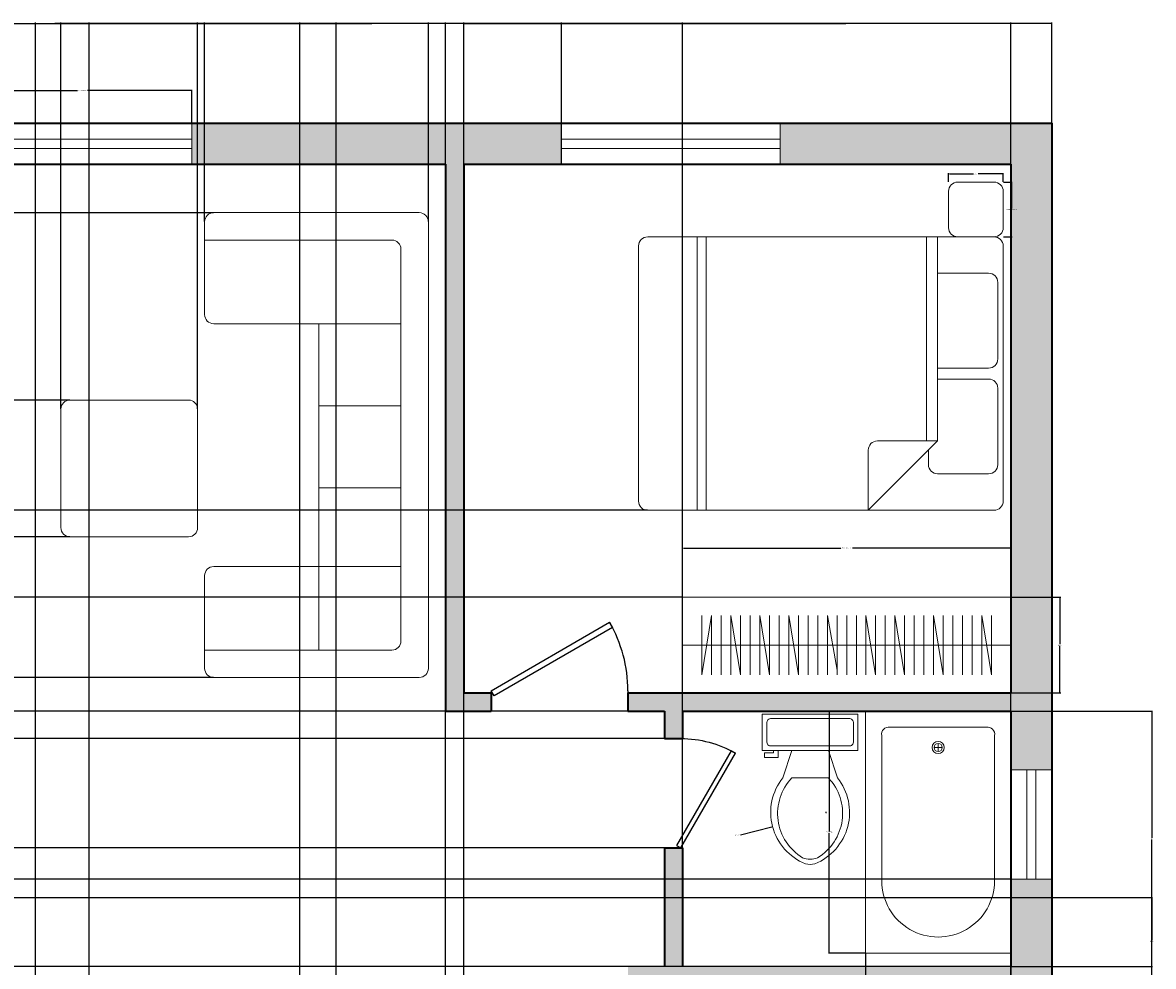
# Model space of a CAD drawing. Units: inches. Extents: x 2800 to 3283, y 1752 to 2114.
# Tile 6 of 6: x 3035 to 3283, y 1907 to 2114. Entities that reach past the tile are written whole.
import ezdxf

# ---------------------------------------------------------------- set-up
doc = ezdxf.new("R2010")
doc.units = ezdxf.units.IN
for name, color, linetype, lineweight in [('A-ANNO-DIMS', 2, 'Continuous', 18), ('A-DOOR', 3, 'Continuous', 25), ('A-FLOR-CASE', 8, 'Continuous', 18), ('A-FLOR-FIXT', 9, 'Continuous', 18), ('A-FURN', 9, 'Continuous', 18), ('A-GLAZ', 4, 'Continuous', 18), ('A-WALL', 7, 'Continuous', 35)]:
    doc.layers.add(name, color=color, linetype=linetype, lineweight=lineweight)
doc.layers.add('A-WALL-PATT', color=18, linetype='Continuous', lineweight=13, true_color=0x000000)
doc.styles.get("Standard").update_dxf_attribs({"font": 'arial.ttf'})
doc.dimstyles.get("Standard").update_dxf_attribs({"dimtxt": 0.18, "dimasz": 0.18, "dimexe": 0.18, "dimexo": 0.0625, "dimgap": 0.09, "dimtad": 0, "dimtih": 1, "dimtoh": 1, "dimdec": 4, "dimzin": 0, "dimdsep": 46, "dimtxsty": 'Standard', "dimcen": 0.09, "dimadec": 0, "dimazin": 0, "dimtfac": 1, "dimtdec": 4, "dimtofl": 0, "dimtmove": 0, "dimatfit": 3, "dimfxl": 1, "dimtolj": 1, "dimtzin": 0, "dimarcsym": 0})

# ---------------------------------------------------------------- blocks, each defined once
blk = doc.blocks.new('Bed - Queen')
for p, q in [((2, 0), (58, 0)), ((0, -78), (0, -2)), ((10, -1.2), (26.8, -1.2)), ((33.2, -1.2), (50, -1.2)), ((60, -2), (60, -78)), ((8, -14.4), (8, -3.2)), ((28.8, -3.2), (28.8, -14.4)), ((31.2, -14.4), (31.2, -3.2)), ((52, -3.2), (52, -14.4)), ((0, -14.4), (44.8, -14.4)), ((60, -29.6), (44.8, -14.4)), ((44.8, -14.4), (44.8, -27.6)), ((44.8, -16.8), (0, -16.8)), ((50, -16.4), (46.8, -16.4)), ((46.8, -29.6), (60, -29.6)), ((0, -65.18), (60, -65.18)), ((0, -67.18), (60, -67.18)), ((58, -80), (2, -80))]:
    blk.add_line(p, q)
for centre, start, end in [((58, -2), 0, 90), ((2, -2), 90, 180), ((10, -3.2), 90, 180), ((26.8, -3.2), 0, 90), ((33.2, -3.2), 90, 180), ((50, -3.2), 0, 90), ((50, -14.4), 270, 0), ((46.8, -27.6), 180, 270), ((2, -78), 180, 270), ((58, -78), 270, 0)]:
    blk.add_arc(centre, 2, start, end)
blk = doc.blocks.new('Bath Tub - 26 x 60 in.')
for p, q in [((8, -18), (10, -18)), ((9, -17), (9, -19))]:
    blk.add_line(p, q)
blk.add_lwpolyline([(0, -36), (0, 0), (60, 0), (60, -36)], close=True)
for points in [[(6, -4), (42, -4)], [(4, -30), (4, -6)], [(42, -32), (6, -32)]]:
    blk.add_lwpolyline(points)
for radius in [1.5, 1]:
    blk.add_circle((9, -18), radius)
for centre, radius, start, end in [((5.75, -5.75), 1.77, 81.8699, 188.1301), ((42, -18), 14, 270, 90), ((5.75, -30.25), 1.77, 171.8699, 278.1301)]:
    blk.add_arc(centre, radius, start, end)
blk = doc.blocks.new('Toilet - top')
for p, q in [((9.5, -6), (9.5, -2)), ((-10, -8.5), (-8, -8.5)), ((-10, -9.5), (-10, -8.5)), ((-7, -9.5), (-10, -9.5)), ((-8, -8.5), (-8, -8)), ((-7, -8), (-7, -9.5)), ((-4, -8), (-6, -14)), ((4, -8), (6, -14)), ((4, -14), (-4, -14))]:
    blk.add_line(p, q)
blk.add_lwpolyline([(10.5, -8), (10.5, 0), (-10.5, 0), (-10.5, -8)], close=True)
for points in [[(-9.5, -2), (-9.5, -6)], [(8.5, -1), (-8.5, -1)], [(-8.5, -7), (8.5, -7)]]:
    blk.add_lwpolyline(points)
for centre, radius, start, end in [((-8.62, -1.88), 0.884, 81.8699, 188.1301), ((8.62, -1.88), 0.884, 351.8699, 98.1301), ((-8.62, -6.12), 0.884, 171.8699, 278.1301), ((8.62, -6.12), 0.884, 261.8699, 8.1301), ((3.52, -21.58), 12.17, 141.4691, 247.9714), ((4.2, -21.82), 11.33, 136.3677, 238.9468), ((-3.52, -21.58), 12.17, 292.0284, 38.5307), ((-4.2, -21.82), 11.33, 301.053, 43.6321), ((0, -27.88), 4, 245.7318, 294.2682), ((0, -29), 4, 254.8605, 285.1395)]:
    blk.add_arc(centre, radius, start, end)
blk = doc.blocks.new('*U12')
for p, q in [((0, 0), (0, -6)), ((40, 0), (40, -6))]:
    blk.add_line(p, q)
blk.add_lwpolyline([(0, 0), (34.64, 20), (35.52, 18.48), (0.87, -1.52)], close=True)
blk.add_arc((0, 0), 40, 0, 30)
blk = doc.blocks.new('WARDROBE-72')
for p, q in [((10.5, 72), (10.5, 0)), ((17, 63.53), (4, 63.53)), ((17, 61.41), (4, 61.41)), ((17, 59.29), (4, 59.29)), ((17, 52.94), (4, 52.94)), ((17, 50.82), (4, 50.82)), ((17, 44.47), (4, 44.47)), ((17, 38.12), (4, 38.12)), ((17, 36), (4, 36)), ((17, 33.88), (4, 33.88)), ((17, 29.65), (4, 29.65)), ((17, 27.53), (4, 27.53)), ((17, 21.18), (4, 21.18)), ((17, 14.82), (4, 14.82)), ((17, 8.47), (4, 8.47))]:
    blk.add_line(p, q)
for points in [[(0, 0), (0, 72), (21, 72), (21, 0), (0, 0), (21, 0)], [(4, 67.76), (17, 67.76), (4, 65.65), (17, 65.65)], [(4, 57.18), (17, 57.18), (4, 55.06), (17, 55.06)], [(4, 48.71), (17, 48.71), (4, 46.59), (17, 46.59)], [(4, 42.35), (17, 42.35), (4, 40.23), (17, 40.23)], [(16.02, 33.88), (4, 31.76), (17, 31.76)], [(4, 25.41), (17, 25.41), (4, 23.29), (17, 23.29)], [(4, 19.06), (17, 19.06), (4, 16.94), (17, 16.94)], [(4, 12.71), (17, 12.71), (4, 10.59), (17, 10.59)], [(4, 4.23), (17, 4.23), (4, 6.35), (17, 6.35)]]:
    blk.add_lwpolyline(points)
blk = doc.blocks.new('WIN-48')
for p, q in [((0, 5.5), (48, 5.5)), ((0, 3.5), (48, 3.5))]:
    blk.add_line(p, q)
for points in [[(0, 0), (0, 9)], [(48, 9), (48, 0)]]:
    blk.add_lwpolyline(points)
blk = doc.blocks.new('WIN-24')
for p, q in [((3.5, 24), (3.5, 0)), ((5.5, 24), (5.5, 0))]:
    blk.add_line(p, q)
for points in [[(0, 24), (9, 24)], [(9, 0), (0, 0)]]:
    blk.add_lwpolyline(points)
blk = doc.blocks.new('NIGHTSTAND-12')
blk.add_lwpolyline([(2, 0), (10, 0, 0.414214), (12, 2), (12, 10, 0.414214), (10, 12), (2, 12, 0.414214), (0, 10), (0, 2, 0.414214)], format="xyb", close=True)
blk = doc.blocks.new('*D19')
at = {"layer": 'A-ANNO-DIMS', "color": 0, "lineweight": -2, "transparency": 16777216}
for p, q in [((3023.88, 2092.33), (3023.88, 2099.65)), ((3024.06, 2099.47), (3046.76, 2099.47)), ((3071.7, 2099.47), (3049, 2099.47)), ((3071.88, 2092.33), (3071.88, 2099.65))]:
    blk.add_line(p, q, dxfattribs=at)
at = {"layer": 'A-ANNO-DIMS', "color": 0, "transparency": 16777216}
for points in [[(3024.06, 2099.5), (3024.06, 2099.44), (3023.88, 2099.47)], [(3071.7, 2099.5), (3071.7, 2099.44), (3071.88, 2099.47)]]:
    blk.add_solid(points, dxfattribs=at)
at = {"layer": 'Defpoints', "color": 0, "transparency": 16777216}
for p in [(3023.88, 2099.47), (3023.88, 2092.27), (3071.88, 2092.27)]:
    blk.add_point(p, dxfattribs=at)
at = {"layer": 'A-ANNO-DIMS', "color": 0, "transparency": 16777216, "insert": (3047.88, 2099.47), "char_height": 0.18, "attachment_point": 5}
blk.add_mtext('\\A1;WINDOW 48 TYP.', dxfattribs=at)
blk = doc.blocks.new('*D25')
at = {"layer": 'A-ANNO-DIMS', "color": 0, "lineweight": -2, "transparency": 16777216}
for p, q in [((3179.54, 1988.33), (3179.54, 1999.25)), ((3179.72, 1999.07), (3214.24, 1999.07)), ((3251.36, 1999.07), (3216.85, 1999.07)), ((3251.54, 1988.33), (3251.54, 1999.25))]:
    blk.add_line(p, q, dxfattribs=at)
at = {"layer": 'A-ANNO-DIMS', "color": 0, "transparency": 16777216}
for points in [[(3179.72, 1999.1), (3179.72, 1999.04), (3179.54, 1999.07)], [(3251.36, 1999.1), (3251.36, 1999.04), (3251.54, 1999.07)]]:
    blk.add_solid(points, dxfattribs=at)
at = {"layer": 'Defpoints', "color": 0, "transparency": 16777216}
for p in [(3251.54, 1999.07), (3179.54, 1988.27), (3251.54, 1988.27)]:
    blk.add_point(p, dxfattribs=at)
at = {"layer": 'A-ANNO-DIMS', "color": 0, "transparency": 16777216, "insert": (3215.54, 1999.07), "char_height": 0.18, "attachment_point": 5}
blk.add_mtext('\\A1;WARDROBE 72 TYP.', dxfattribs=at)
blk = doc.blocks.new('*D26')
at = {"layer": 'A-ANNO-DIMS', "color": 0, "lineweight": -2, "transparency": 16777216}
for p, q in [((3251.61, 1988.27), (3262.52, 1988.27)), ((3262.34, 1988.09), (3262.34, 1977.95)), ((3262.34, 1967.45), (3262.34, 1977.59)), ((3251.61, 1967.27), (3262.52, 1967.27))]:
    blk.add_line(p, q, dxfattribs=at)
at = {"layer": 'A-ANNO-DIMS', "color": 0, "transparency": 16777216}
for points in [[(3262.31, 1988.09), (3262.37, 1988.09), (3262.34, 1988.27)], [(3262.31, 1967.45), (3262.37, 1967.45), (3262.34, 1967.27)]]:
    blk.add_solid(points, dxfattribs=at)
at = {"layer": 'Defpoints', "color": 0, "transparency": 16777216}
for p in [(3251.54, 1988.27), (3251.54, 1967.27), (3262.34, 1967.27)]:
    blk.add_point(p, dxfattribs=at)
at = {"layer": 'A-ANNO-DIMS', "color": 0, "transparency": 16777216, "insert": (3262.34, 1977.77), "char_height": 0.18, "attachment_point": 5}
blk.add_mtext('\\A1;21 TYP.', dxfattribs=at)
blk = doc.blocks.new('*D29')
at = {"layer": 'A-ANNO-DIMS', "color": 0, "lineweight": -2, "transparency": 16777216}
for p, q in [((3249.95, 2079.36), (3251.87, 2079.36)), ((3251.69, 2079.18), (3251.69, 2073.54)), ((3251.69, 2067.54), (3251.69, 2073.18)), ((3249.95, 2067.36), (3251.87, 2067.36))]:
    blk.add_line(p, q, dxfattribs=at)
at = {"layer": 'A-ANNO-DIMS', "color": 0, "transparency": 16777216}
for points in [[(3251.66, 2079.18), (3251.72, 2079.18), (3251.69, 2079.36)], [(3251.66, 2067.54), (3251.72, 2067.54), (3251.69, 2067.36)]]:
    blk.add_solid(points, dxfattribs=at)
at = {"layer": 'Defpoints', "color": 0, "transparency": 16777216}
for p in [(3249.89, 2079.36), (3251.69, 2079.36), (3249.89, 2067.36)]:
    blk.add_point(p, dxfattribs=at)
at = {"layer": 'A-ANNO-DIMS', "color": 0, "transparency": 16777216, "insert": (3251.69, 2073.36), "char_height": 0.18, "attachment_point": 5}
blk.add_mtext('\\A1;NIGHTSTAND 12 TYP.', dxfattribs=at)
blk = doc.blocks.new('*D30')
at = {"layer": 'A-ANNO-DIMS', "color": 0, "lineweight": -2, "transparency": 16777216}
for p, q in [((3237.89, 2079.42), (3237.89, 2081.34)), ((3238.07, 2081.16), (3243.37, 2081.16)), ((3249.71, 2081.16), (3244.41, 2081.16)), ((3249.89, 2079.42), (3249.89, 2081.34))]:
    blk.add_line(p, q, dxfattribs=at)
at = {"layer": 'A-ANNO-DIMS', "color": 0, "transparency": 16777216}
for points in [[(3238.07, 2081.19), (3238.07, 2081.13), (3237.89, 2081.16)], [(3249.71, 2081.19), (3249.71, 2081.13), (3249.89, 2081.16)]]:
    blk.add_solid(points, dxfattribs=at)
at = {"layer": 'Defpoints', "color": 0, "transparency": 16777216}
for p in [(3237.89, 2081.16), (3237.89, 2079.36), (3249.89, 2079.36)]:
    blk.add_point(p, dxfattribs=at)
at = {"layer": 'A-ANNO-DIMS', "color": 0, "transparency": 16777216, "insert": (3243.89, 2081.16), "char_height": 0.18, "attachment_point": 5}
blk.add_mtext('\\A1;12 TYP.', dxfattribs=at)
blk = doc.blocks.new('*D31')
at = {"layer": 'A-ANNO-DIMS', "color": 0, "lineweight": -2, "transparency": 16777216}
for p, q in [((3219.62, 1963.27), (3211.53, 1963.27)), ((3211.71, 1963.09), (3211.71, 1936.9)), ((3211.71, 1910.34), (3211.71, 1936.53)), ((3219.62, 1910.16), (3211.53, 1910.16))]:
    blk.add_line(p, q, dxfattribs=at)
at = {"layer": 'A-ANNO-DIMS', "color": 0, "transparency": 16777216}
for points in [[(3211.68, 1963.09), (3211.74, 1963.09), (3211.71, 1963.27)], [(3211.68, 1910.34), (3211.74, 1910.34), (3211.71, 1910.16)]]:
    blk.add_solid(points, dxfattribs=at)
at = {"layer": 'Defpoints', "color": 0, "transparency": 16777216}
for p in [(3219.68, 1963.27), (3211.71, 1910.16), (3219.68, 1910.16)]:
    blk.add_point(p, dxfattribs=at)
at = {"layer": 'A-ANNO-DIMS', "color": 0, "transparency": 16777216, "insert": (3211.71, 1936.72), "char_height": 0.18, "attachment_point": 5}
blk.add_mtext('\\A1;TUB 53 TYP.', dxfattribs=at)
blk = doc.blocks.new('*D32')
at = {"layer": 'A-ANNO-DIMS', "color": 0, "lineweight": -2, "transparency": 16777216}
for p, q in [((3219.68, 1910.1), (3219.68, 1902.02)), ((3251.54, 1910.1), (3251.54, 1902.02)), ((3219.86, 1902.2), (3235.08, 1902.2)), ((3251.36, 1902.2), (3236.14, 1902.2))]:
    blk.add_line(p, q, dxfattribs=at)
at = {"layer": 'A-ANNO-DIMS', "color": 0, "transparency": 16777216}
for points in [[(3219.86, 1902.23), (3219.86, 1902.17), (3219.68, 1902.2)], [(3251.36, 1902.23), (3251.36, 1902.17), (3251.54, 1902.2)]]:
    blk.add_solid(points, dxfattribs=at)
at = {"layer": 'Defpoints', "color": 0, "transparency": 16777216}
for p in [(3219.68, 1910.16), (3251.54, 1910.16), (3251.54, 1902.2)]:
    blk.add_point(p, dxfattribs=at)
at = {"layer": 'A-ANNO-DIMS', "color": 0, "transparency": 16777216, "insert": (3235.61, 1902.2), "char_height": 0.18, "attachment_point": 5}
blk.add_mtext('\\A1;32 TYP.', dxfattribs=at)
blk = doc.blocks.new('*D43')
at = {"layer": 'A-ANNO-DIMS', "color": 0, "lineweight": -2, "transparency": 16777216}
for p, q in [((2822.54, 2092.33), (2822.54, 2114.36)), ((2822.72, 2114.18), (3041.25, 2114.18)), ((3260.36, 2114.18), (3041.84, 2114.18)), ((3260.54, 2092.33), (3260.54, 2114.36))]:
    blk.add_line(p, q, dxfattribs=at)
at = {"layer": 'A-ANNO-DIMS', "color": 0, "transparency": 16777216}
for points in [[(2822.72, 2114.21), (2822.72, 2114.15), (2822.54, 2114.18)], [(3260.36, 2114.21), (3260.36, 2114.15), (3260.54, 2114.18)]]:
    blk.add_solid(points, dxfattribs=at)
at = {"layer": 'Defpoints', "color": 0, "transparency": 16777216}
for p in [(3260.54, 2114.18), (2822.54, 2092.27), (3260.54, 2092.27)]:
    blk.add_point(p, dxfattribs=at)
at = {"layer": 'A-ANNO-DIMS', "color": 0, "transparency": 16777216, "insert": (3041.54, 2114.18), "char_height": 0.18, "attachment_point": 5}
blk.add_mtext('\\A1;438', dxfattribs=at)
blk = doc.blocks.new('*D47')
at = {"layer": 'A-ANNO-DIMS', "color": 0, "lineweight": -2, "transparency": 16777216}
for p, q in [((2955.54, 1963.33), (2955.54, 2114.36)), ((2955.72, 2114.18), (3041.26, 2114.18)), ((3127.36, 2114.18), (3041.82, 2114.18)), ((3127.54, 1963.33), (3127.54, 2114.36))]:
    blk.add_line(p, q, dxfattribs=at)
at = {"layer": 'A-ANNO-DIMS', "color": 0, "transparency": 16777216}
for points in [[(2955.72, 2114.21), (2955.72, 2114.15), (2955.54, 2114.18)], [(3127.36, 2114.21), (3127.36, 2114.15), (3127.54, 2114.18)]]:
    blk.add_solid(points, dxfattribs=at)
at = {"layer": 'Defpoints', "color": 0, "transparency": 16777216}
for p in [(3127.54, 2114.18), (2955.54, 1963.27), (3127.54, 1963.27)]:
    blk.add_point(p, dxfattribs=at)
at = {"layer": 'A-ANNO-DIMS', "color": 0, "transparency": 16777216, "insert": (3041.54, 2114.18), "char_height": 0.18, "attachment_point": 5}
blk.add_mtext('\\A1;172', dxfattribs=at)
blk = doc.blocks.new('*D48')
at = {"layer": 'A-ANNO-DIMS', "color": 0, "lineweight": -2, "transparency": 16777216}
for p, q in [((3131.54, 1783.33), (3131.54, 2114.36)), ((3131.72, 2114.18), (3191.26, 2114.18)), ((3251.36, 2114.18), (3191.82, 2114.18)), ((3251.54, 1783.33), (3251.54, 2114.36))]:
    blk.add_line(p, q, dxfattribs=at)
at = {"layer": 'A-ANNO-DIMS', "color": 0, "transparency": 16777216}
for points in [[(3131.72, 2114.21), (3131.72, 2114.15), (3131.54, 2114.18)], [(3251.36, 2114.21), (3251.36, 2114.15), (3251.54, 2114.18)]]:
    blk.add_solid(points, dxfattribs=at)
at = {"layer": 'Defpoints', "color": 0, "transparency": 16777216}
for p in [(3251.54, 2114.18), (3131.54, 1783.27), (3251.54, 1783.27)]:
    blk.add_point(p, dxfattribs=at)
at = {"layer": 'A-ANNO-DIMS', "color": 0, "transparency": 16777216, "insert": (3191.54, 2114.18), "char_height": 0.18, "attachment_point": 5}
blk.add_mtext('\\A1;120', dxfattribs=at)
blk = doc.blocks.new('*D52')
at = {"layer": 'A-ANNO-DIMS', "color": 0, "lineweight": -2, "transparency": 16777216}
for p, q in [((3251.61, 1963.27), (3282.64, 1963.27)), ((3282.46, 1963.09), (3282.46, 1935.45)), ((3282.46, 1907.45), (3282.46, 1935.09)), ((3251.61, 1907.27), (3282.64, 1907.27))]:
    blk.add_line(p, q, dxfattribs=at)
at = {"layer": 'A-ANNO-DIMS', "color": 0, "transparency": 16777216}
for points in [[(3282.43, 1963.09), (3282.49, 1963.09), (3282.46, 1963.27)], [(3282.43, 1907.45), (3282.49, 1907.45), (3282.46, 1907.27)]]:
    blk.add_solid(points, dxfattribs=at)
at = {"layer": 'Defpoints', "color": 0, "transparency": 16777216}
for p in [(3251.54, 1963.27), (3282.46, 1963.27), (3251.54, 1907.27)]:
    blk.add_point(p, dxfattribs=at)
at = {"layer": 'A-ANNO-DIMS', "color": 0, "transparency": 16777216, "insert": (3282.46, 1935.27), "char_height": 0.18, "attachment_point": 5}
blk.add_mtext('\\A1;56', dxfattribs=at)
blk = doc.blocks.new('*D55')
at = {"layer": 'A-ANNO-DIMS', "color": 0, "lineweight": -2, "transparency": 16777216}
for p, q in [((3179.54, 1907.33), (3179.54, 2114.36)), ((3179.72, 2114.18), (3215.33, 2114.18)), ((3251.36, 2114.18), (3215.76, 2114.18)), ((3251.54, 1907.33), (3251.54, 2114.36))]:
    blk.add_line(p, q, dxfattribs=at)
at = {"layer": 'A-ANNO-DIMS', "color": 0, "transparency": 16777216}
for points in [[(3179.72, 2114.21), (3179.72, 2114.15), (3179.54, 2114.18)], [(3251.36, 2114.21), (3251.36, 2114.15), (3251.54, 2114.18)]]:
    blk.add_solid(points, dxfattribs=at)
at = {"layer": 'Defpoints', "color": 0, "transparency": 16777216}
for p in [(3251.54, 2114.18), (3179.54, 1907.27), (3251.54, 1907.27)]:
    blk.add_point(p, dxfattribs=at)
at = {"layer": 'A-ANNO-DIMS', "color": 0, "transparency": 16777216, "insert": (3215.54, 2114.18), "char_height": 0.18, "attachment_point": 5}
blk.add_mtext('\\A1;72', dxfattribs=at)
blk = doc.blocks.new('*D58')
at = {"layer": 'A-ANNO-DIMS', "color": 0, "lineweight": -2, "transparency": 16777216}
for p, q in [((3131.54, 2083.33), (3131.54, 2114.36)), ((3131.72, 2114.18), (3141.87, 2114.18)), ((3152.77, 2114.18), (3142.63, 2114.18)), ((3152.95, 2083.33), (3152.95, 2114.36))]:
    blk.add_line(p, q, dxfattribs=at)
at = {"layer": 'A-ANNO-DIMS', "color": 0, "transparency": 16777216}
for points in [[(3131.72, 2114.21), (3131.72, 2114.15), (3131.54, 2114.18)], [(3152.77, 2114.21), (3152.77, 2114.15), (3152.95, 2114.18)]]:
    blk.add_solid(points, dxfattribs=at)
at = {"layer": 'Defpoints', "color": 0, "transparency": 16777216}
for p in [(3152.95, 2114.18), (3131.54, 2083.27), (3152.95, 2083.27)]:
    blk.add_point(p, dxfattribs=at)
at = {"layer": 'A-ANNO-DIMS', "color": 0, "transparency": 16777216, "insert": (3142.25, 2114.18), "char_height": 0.18, "attachment_point": 5}
blk.add_mtext('\\A1;21.41', dxfattribs=at)
blk = doc.blocks.new('*D64')
at = {"layer": 'A-ANNO-DIMS', "color": 0, "lineweight": -2, "transparency": 16777216}
for p, q in [((2831.61, 1922.35), (3282.64, 1922.35)), ((3282.46, 1922.17), (3282.46, 1912.99)), ((3282.46, 1903.45), (3282.46, 1912.63)), ((2831.61, 1903.27), (3282.64, 1903.27))]:
    blk.add_line(p, q, dxfattribs=at)
at = {"layer": 'A-ANNO-DIMS', "color": 0, "transparency": 16777216}
for points in [[(3282.43, 1922.17), (3282.49, 1922.17), (3282.46, 1922.35)], [(3282.43, 1903.45), (3282.49, 1903.45), (3282.46, 1903.27)]]:
    blk.add_solid(points, dxfattribs=at)
at = {"layer": 'Defpoints', "color": 0, "transparency": 16777216}
for p in [(2831.54, 1922.35), (3282.46, 1922.35), (2831.54, 1903.27)]:
    blk.add_point(p, dxfattribs=at)
at = {"layer": 'A-ANNO-DIMS', "color": 0, "transparency": 16777216, "insert": (3282.46, 1912.81), "char_height": 0.18, "attachment_point": 5}
blk.add_mtext('\\A1;19.085', dxfattribs=at)
blk = doc.blocks.new('*D65')
at = {"layer": 'A-ANNO-DIMS', "color": 0, "lineweight": -2, "transparency": 16777216}
for p, q in [((3251.48, 1926.4), (2800.45, 1926.4)), ((2800.63, 1926.22), (2800.63, 1917.02)), ((2800.63, 1907.45), (2800.63, 1916.65)), ((3251.48, 1907.27), (2800.45, 1907.27))]:
    blk.add_line(p, q, dxfattribs=at)
at = {"layer": 'A-ANNO-DIMS', "color": 0, "transparency": 16777216}
for points in [[(2800.6, 1926.22), (2800.66, 1926.22), (2800.63, 1926.4)], [(2800.6, 1907.45), (2800.66, 1907.45), (2800.63, 1907.27)]]:
    blk.add_solid(points, dxfattribs=at)
at = {"layer": 'Defpoints', "color": 0, "transparency": 16777216}
for p in [(2800.63, 1926.4), (3251.54, 1926.4), (3251.54, 1907.27)]:
    blk.add_point(p, dxfattribs=at)
at = {"layer": 'A-ANNO-DIMS', "color": 0, "transparency": 16777216, "insert": (2800.63, 1916.83), "char_height": 0.18, "attachment_point": 5}
blk.add_mtext('\\A1;19.128', dxfattribs=at)
blk = doc.blocks.new('*D68')
at = {"layer": 'A-ANNO-DIMS', "color": 0, "lineweight": -2, "transparency": 16777216}
for p, q in [((3175.48, 1957.27), (2800.45, 1957.27)), ((2800.63, 1957.09), (2800.63, 1945.45)), ((2800.63, 1933.45), (2800.63, 1945.09)), ((3175.48, 1933.27), (2800.45, 1933.27))]:
    blk.add_line(p, q, dxfattribs=at)
at = {"layer": 'A-ANNO-DIMS', "color": 0, "transparency": 16777216}
for points in [[(2800.6, 1957.09), (2800.66, 1957.09), (2800.63, 1957.27)], [(2800.6, 1933.45), (2800.66, 1933.45), (2800.63, 1933.27)]]:
    blk.add_solid(points, dxfattribs=at)
at = {"layer": 'Defpoints', "color": 0, "transparency": 16777216}
for p in [(2800.63, 1957.27), (3175.54, 1957.27), (3175.54, 1933.27)]:
    blk.add_point(p, dxfattribs=at)
at = {"layer": 'A-ANNO-DIMS', "color": 0, "transparency": 16777216, "insert": (2800.63, 1945.27), "char_height": 0.18, "attachment_point": 5}
blk.add_mtext('\\A1;24', dxfattribs=at)
blk = doc.blocks.new('*D69')
at = {"layer": 'A-ANNO-DIMS', "color": 0, "lineweight": -2, "transparency": 16777216}
for p, q in [((3175.48, 1963.27), (2800.45, 1963.27)), ((2800.63, 1963.09), (2800.63, 1960.45)), ((2800.63, 1957.45), (2800.63, 1960.09)), ((3175.48, 1957.27), (2800.45, 1957.27))]:
    blk.add_line(p, q, dxfattribs=at)
at = {"layer": 'A-ANNO-DIMS', "color": 0, "transparency": 16777216}
for points in [[(2800.6, 1963.09), (2800.66, 1963.09), (2800.63, 1963.27)], [(2800.6, 1957.45), (2800.66, 1957.45), (2800.63, 1957.27)]]:
    blk.add_solid(points, dxfattribs=at)
at = {"layer": 'Defpoints', "color": 0, "transparency": 16777216}
for p in [(2800.63, 1963.27), (3175.54, 1963.27), (3175.54, 1957.27)]:
    blk.add_point(p, dxfattribs=at)
at = {"layer": 'A-ANNO-DIMS', "color": 0, "transparency": 16777216, "insert": (2800.63, 1960.27), "char_height": 0.18, "attachment_point": 5}
blk.add_mtext('\\A1;6', dxfattribs=at)
blk = doc.blocks.new('*D70')
at = {"layer": 'A-ANNO-DIMS', "color": 0, "lineweight": -2, "transparency": 16777216}
for p, q in [((3037.54, 1903.33), (3037.54, 2114.36)), ((3037.72, 2114.18), (3082.32, 2114.18)), ((3127.36, 2114.18), (3082.76, 2114.18)), ((3127.54, 1899.33), (3127.54, 2114.36))]:
    blk.add_line(p, q, dxfattribs=at)
at = {"layer": 'A-ANNO-DIMS', "color": 0, "transparency": 16777216}
for points in [[(3037.72, 2114.21), (3037.72, 2114.15), (3037.54, 2114.18)], [(3127.36, 2114.21), (3127.36, 2114.15), (3127.54, 2114.18)]]:
    blk.add_solid(points, dxfattribs=at)
at = {"layer": 'Defpoints', "color": 0, "transparency": 16777216}
for p in [(3127.54, 2114.18), (3037.54, 1903.27), (3127.54, 1899.27)]:
    blk.add_point(p, dxfattribs=at)
at = {"layer": 'A-ANNO-DIMS', "color": 0, "transparency": 16777216, "insert": (3082.54, 2114.18), "char_height": 0.18, "attachment_point": 5}
blk.add_mtext('\\A1;90', dxfattribs=at)
blk = doc.blocks.new('*D72')
at = {"layer": 'A-ANNO-DIMS', "color": 0, "lineweight": -2, "transparency": 16777216}
for p, q in [((3049.36, 1879.34), (3049.36, 2114.36)), ((3049.54, 2114.18), (3076.06, 2114.18)), ((3103.36, 2114.18), (3076.84, 2114.18)), ((3103.54, 1879.4), (3103.54, 2114.36))]:
    blk.add_line(p, q, dxfattribs=at)
at = {"layer": 'A-ANNO-DIMS', "color": 0, "transparency": 16777216}
for points in [[(3049.54, 2114.21), (3049.54, 2114.15), (3049.36, 2114.18)], [(3103.36, 2114.21), (3103.36, 2114.15), (3103.54, 2114.18)]]:
    blk.add_solid(points, dxfattribs=at)
at = {"layer": 'Defpoints', "color": 0, "transparency": 16777216}
for p in [(3103.54, 2114.18), (3049.36, 1879.28), (3103.54, 1879.34)]:
    blk.add_point(p, dxfattribs=at)
at = {"layer": 'A-ANNO-DIMS', "color": 0, "transparency": 16777216, "insert": (3076.45, 2114.18), "char_height": 0.18, "attachment_point": 5}
blk.add_mtext('\\A1;54.19', dxfattribs=at)
blk = doc.blocks.new('*D74')
at = {"layer": 'A-ANNO-DIMS', "color": 0, "lineweight": -2, "transparency": 16777216}
for p, q in [((3037.54, 1855.51), (3037.54, 2114.36)), ((3037.72, 2114.18), (3043, 2114.18)), ((3049.18, 2114.18), (3043.91, 2114.18)), ((3049.36, 1855.51), (3049.36, 2114.36))]:
    blk.add_line(p, q, dxfattribs=at)
at = {"layer": 'A-ANNO-DIMS', "color": 0, "transparency": 16777216}
for points in [[(3037.72, 2114.21), (3037.72, 2114.15), (3037.54, 2114.18)], [(3049.18, 2114.21), (3049.18, 2114.15), (3049.36, 2114.18)]]:
    blk.add_solid(points, dxfattribs=at)
at = {"layer": 'Defpoints', "color": 0, "transparency": 16777216}
for p in [(3049.36, 2114.18), (3037.54, 1855.45), (3049.36, 1855.45)]:
    blk.add_point(p, dxfattribs=at)
at = {"layer": 'A-ANNO-DIMS', "color": 0, "transparency": 16777216, "insert": (3043.45, 2114.18), "char_height": 0.18, "attachment_point": 5}
blk.add_mtext('\\A1;11.814', dxfattribs=at)
blk = doc.blocks.new('*D75')
at = {"layer": 'A-ANNO-DIMS', "color": 0, "lineweight": -2, "transparency": 16777216}
for p, q in [((3095.54, 1899.33), (3095.54, 2114.36)), ((3095.72, 2114.18), (3111.33, 2114.18)), ((3127.36, 2114.18), (3111.76, 2114.18)), ((3127.54, 1899.33), (3127.54, 2114.36))]:
    blk.add_line(p, q, dxfattribs=at)
at = {"layer": 'A-ANNO-DIMS', "color": 0, "transparency": 16777216}
for points in [[(3095.72, 2114.21), (3095.72, 2114.15), (3095.54, 2114.18)], [(3127.36, 2114.21), (3127.36, 2114.15), (3127.54, 2114.18)]]:
    blk.add_solid(points, dxfattribs=at)
at = {"layer": 'Defpoints', "color": 0, "transparency": 16777216}
for p in [(3127.54, 2114.18), (3095.54, 1899.27), (3127.54, 1899.27)]:
    blk.add_point(p, dxfattribs=at)
at = {"layer": 'A-ANNO-DIMS', "color": 0, "transparency": 16777216, "insert": (3111.54, 2114.18), "char_height": 0.18, "attachment_point": 5}
blk.add_mtext('\\A1;32', dxfattribs=at)
blk = doc.blocks.new('*D77')
at = {"layer": 'A-ANNO-DIMS', "color": 0, "lineweight": -2, "transparency": 16777216}
for p, q in [((3076.62, 2072.66), (2800.45, 2072.66)), ((2800.63, 2072.48), (2800.63, 2021.84)), ((2800.63, 1970.84), (2800.63, 2021.48)), ((3076.62, 1970.66), (2800.45, 1970.66))]:
    blk.add_line(p, q, dxfattribs=at)
at = {"layer": 'A-ANNO-DIMS', "color": 0, "transparency": 16777216}
for points in [[(2800.6, 2072.48), (2800.66, 2072.48), (2800.63, 2072.66)], [(2800.6, 1970.84), (2800.66, 1970.84), (2800.63, 1970.66)]]:
    blk.add_solid(points, dxfattribs=at)
at = {"layer": 'Defpoints', "color": 0, "transparency": 16777216}
for p in [(3076.68, 2072.66), (2800.63, 1970.66), (3076.68, 1970.66)]:
    blk.add_point(p, dxfattribs=at)
at = {"layer": 'A-ANNO-DIMS', "color": 0, "transparency": 16777216, "insert": (2800.63, 2021.66), "char_height": 0.18, "attachment_point": 5}
blk.add_mtext('\\A1;102', dxfattribs=at)
blk = doc.blocks.new('*D78')
at = {"layer": 'A-ANNO-DIMS', "color": 0, "lineweight": -2, "transparency": 16777216}
for p, q in [((3074.68, 2070.72), (3074.68, 2114.36)), ((3074.86, 2114.18), (3098.82, 2114.18)), ((3123.58, 2114.18), (3099.62, 2114.18)), ((3123.76, 2070.72), (3123.76, 2114.36))]:
    blk.add_line(p, q, dxfattribs=at)
at = {"layer": 'A-ANNO-DIMS', "color": 0, "transparency": 16777216}
for points in [[(3074.86, 2114.21), (3074.86, 2114.15), (3074.68, 2114.18)], [(3123.58, 2114.21), (3123.58, 2114.15), (3123.76, 2114.18)]]:
    blk.add_solid(points, dxfattribs=at)
at = {"layer": 'Defpoints', "color": 0, "transparency": 16777216}
for p in [(3123.76, 2114.18), (3074.68, 2070.66), (3123.76, 2070.66)]:
    blk.add_point(p, dxfattribs=at)
at = {"layer": 'A-ANNO-DIMS', "color": 0, "transparency": 16777216, "insert": (3099.22, 2114.18), "char_height": 0.18, "attachment_point": 5}
blk.add_mtext('\\A1;49.08', dxfattribs=at)
blk = doc.blocks.new('*D79')
at = {"layer": 'A-ANNO-DIMS', "color": 0, "lineweight": -2, "transparency": 16777216}
for p, q in [((3043.14, 2029.61), (3043.14, 2114.36)), ((3043.32, 2114.18), (3057.92, 2114.18)), ((3072.96, 2114.18), (3058.36, 2114.18)), ((3073.14, 2029.61), (3073.14, 2114.36))]:
    blk.add_line(p, q, dxfattribs=at)
at = {"layer": 'A-ANNO-DIMS', "color": 0, "transparency": 16777216}
for points in [[(3043.32, 2114.21), (3043.32, 2114.15), (3043.14, 2114.18)], [(3072.96, 2114.21), (3072.96, 2114.15), (3073.14, 2114.18)]]:
    blk.add_solid(points, dxfattribs=at)
at = {"layer": 'Defpoints', "color": 0, "transparency": 16777216}
for p in [(3073.14, 2114.18), (3043.14, 2029.54), (3073.14, 2029.54)]:
    blk.add_point(p, dxfattribs=at)
at = {"layer": 'A-ANNO-DIMS', "color": 0, "transparency": 16777216, "insert": (3058.14, 2114.18), "char_height": 0.18, "attachment_point": 5}
blk.add_mtext('\\A1;30', dxfattribs=at)
blk = doc.blocks.new('*D80')
at = {"layer": 'A-ANNO-DIMS', "color": 0, "lineweight": -2, "transparency": 16777216}
for p, q in [((3045.08, 2031.54), (2800.45, 2031.54)), ((2800.63, 2031.36), (2800.63, 2016.73)), ((2800.63, 2001.72), (2800.63, 2016.36)), ((3045.08, 2001.54), (2800.45, 2001.54))]:
    blk.add_line(p, q, dxfattribs=at)
at = {"layer": 'A-ANNO-DIMS', "color": 0, "transparency": 16777216}
for points in [[(2800.6, 2031.36), (2800.66, 2031.36), (2800.63, 2031.54)], [(2800.6, 2001.72), (2800.66, 2001.72), (2800.63, 2001.54)]]:
    blk.add_solid(points, dxfattribs=at)
at = {"layer": 'Defpoints', "color": 0, "transparency": 16777216}
for p in [(2800.63, 2031.54), (3045.14, 2031.54), (3045.14, 2001.54)]:
    blk.add_point(p, dxfattribs=at)
at = {"layer": 'A-ANNO-DIMS', "color": 0, "transparency": 16777216, "insert": (2800.63, 2016.54), "char_height": 0.18, "attachment_point": 5}
blk.add_mtext('\\A1;30', dxfattribs=at)
blk = doc.blocks.new('*D82')
at = {"layer": 'A-ANNO-DIMS', "color": 0, "lineweight": -2, "transparency": 16777216}
for p, q in [((3171.82, 2007.36), (2800.45, 2007.36)), ((2800.63, 2007.18), (2800.63, 1998)), ((2800.63, 1988.45), (2800.63, 1997.63)), ((3179.48, 1988.27), (2800.45, 1988.27))]:
    blk.add_line(p, q, dxfattribs=at)
at = {"layer": 'A-ANNO-DIMS', "color": 0, "transparency": 16777216}
for points in [[(2800.6, 2007.18), (2800.66, 2007.18), (2800.63, 2007.36)], [(2800.6, 1988.45), (2800.66, 1988.45), (2800.63, 1988.27)]]:
    blk.add_solid(points, dxfattribs=at)
at = {"layer": 'Defpoints', "color": 0, "transparency": 16777216}
for p in [(2800.63, 2007.36), (3171.89, 2007.36), (3179.54, 1988.27)]:
    blk.add_point(p, dxfattribs=at)
at = {"layer": 'A-ANNO-DIMS', "color": 0, "transparency": 16777216, "insert": (2800.63, 1997.81), "char_height": 0.18, "attachment_point": 5}
blk.add_mtext('\\A1;19.09', dxfattribs=at)
blk = doc.blocks.new('*D88')
at = {"layer": 'A-ANNO-DIMS', "color": 0, "lineweight": -2, "transparency": 16777216}
for p, q in [((3210.95, 1941.06), (3211.13, 1941.06)), ((3211.04, 1940.97), (3211.04, 1941.15)), ((3192.21, 1936.11), (3199.1, 1937.92))]:
    blk.add_line(p, q, dxfattribs=at)
at = {"layer": 'A-ANNO-DIMS', "color": 0, "transparency": 16777216}
blk.add_solid([(3199.09, 1937.95), (3199.1, 1937.89), (3199.27, 1937.97)], dxfattribs=at)
at = {"layer": 'Defpoints', "color": 0, "transparency": 16777216}
for p in [(3211.04, 1941.06), (3199.27, 1937.97)]:
    blk.add_point(p, dxfattribs=at)
at = {"layer": 'A-ANNO-DIMS', "color": 0, "transparency": 16777216, "insert": (3191.53, 1936.11), "char_height": 0.18, "attachment_point": 5}
blk.add_mtext('\\A1;4X R12.17', dxfattribs=at)

msp = doc.modelspace()

# ---------------------------------------------------------------- hatches: boundary and pattern name
at = {"layer": 'A-WALL-PATT'}
h = msp.add_hatch(color=256, dxfattribs=at)
h.dxf.hatch_style = 1
h.paths.add_polyline_path([(3152.9512, 2092.2695), (3071.883, 2092.2695), (3071.883, 2083.2695), (3127.5432, 2083.2695), (3127.5432, 1963.2695), (3137.5432, 1963.2695), (3137.5432, 1967.2695), (3131.5432, 1967.2695), (3131.5432, 2083.2695), (3152.9512, 2083.2695)])
h = msp.add_hatch(color=256, dxfattribs=at)
h.dxf.hatch_style = 1
h.paths.add_polyline_path([(3260.5432, 2092.2695), (3200.9512, 2092.2695), (3200.9512, 2083.2695), (3251.5432, 2083.2695), (3251.5432, 1967.2695), (3179.5432, 1967.2695), (3167.5432, 1967.2695), (3167.5432, 1963.2695), (3175.5432, 1963.2695), (3175.5432, 1957.2695), (3179.5432, 1957.2695), (3179.5432, 1963.2695), (3251.5432, 1963.2695), (3251.5432, 1950.3971), (3260.5432, 1950.3971)])
h = msp.add_hatch(color=256, dxfattribs=at)
h.dxf.hatch_style = 1
h.paths.add_polyline_path([(3260.5432, 1926.3971), (3251.5432, 1926.3971), (3251.5432, 1910.1641), (3251.5432, 1907.2695), (3179.5432, 1907.2695), (3179.5432, 1933.2695), (3175.5432, 1933.2695), (3175.5432, 1907.2695), (3167.5432, 1907.2695), (3167.5432, 1903.2695), (3251.5432, 1903.2695), (3251.5432, 1882.2695), (3251.5432, 1783.2695), (3197.6001, 1783.2695), (3197.6001, 1774.2695), (3260.5432, 1774.2695)])

# ---------------------------------------------------------------- linework, layer by layer
at = {"layer": 'A-FURN'}
for p, q in [((3076.6778, 2072.661), (3121.7585, 2072.661)), ((3074.6778, 2066.661), (3074.6778, 2070.661)), ((3123.7585, 2070.661), (3123.7585, 1972.661)), ((3074.6778, 2066.661), (3115.7585, 2066.661)), ((3117.7585, 2064.661), (3117.7585, 1978.661)), ((3099.7585, 1995.0215), (3099.7585, 1976.661)), ((3115.7585, 1976.661), (3074.6778, 1976.661)), ((3074.6778, 1976.661), (3074.6778, 1972.661)), ((3121.7585, 1970.661), (3076.6778, 1970.661))]:
    msp.add_line(p, q, dxfattribs=at)
for points in [[(3115.7585, 2066.661), (3074.6778, 2066.661), (3074.6778, 2050.3005, 0.41421356), (3076.6778, 2048.3005), (3117.7585, 2048.3005), (3117.7585, 2064.661, 0.41421356)], [(3071.1406, 2031.544), (3045.1406, 2031.544, 0.41421356), (3043.1406, 2029.544), (3043.1406, 2003.544, 0.41421356), (3045.1406, 2001.544), (3071.1406, 2001.544, 0.41421356), (3073.1406, 2003.544), (3073.1406, 2029.544, 0.41421356)], [(3117.7585, 1995.0215), (3076.6778, 1995.0215, 0.41421356), (3074.6778, 1993.0215), (3074.6778, 1976.661), (3115.7585, 1976.661, 0.41421356), (3117.7585, 1978.661)]]:
    msp.add_lwpolyline(points, format="xyb", close=True, dxfattribs=at)
for points in [[(3117.7585, 2048.3005), (3099.7585, 2048.3005), (3099.7585, 2030.3005), (3117.7585, 2030.3005)], [(3117.7585, 2030.3005), (3099.7585, 2030.3005), (3099.7585, 2012.3005), (3117.7585, 2012.3005)]]:
    msp.add_lwpolyline(points, close=True, dxfattribs=at)
msp.add_lwpolyline([(3117.7585, 1994.3005), (3117.7585, 2012.3005), (3099.7585, 2012.3005), (3099.7585, 1995.0215)], dxfattribs=at)
for centre, start, end in [((3076.6778, 2070.661), 90, 180), ((3121.7585, 2070.661), 0, 90), ((3115.7585, 2064.661), 0, 90), ((3115.7585, 1978.661), 270, 0), ((3076.6778, 1972.661), 180, 270), ((3121.7585, 1972.661), 270, 0)]:
    msp.add_arc(centre, 2, start, end, dxfattribs=at)
at = {"layer": 'A-WALL'}
for p, q in [((2955.5432, 2083.2695), (3127.5432, 2083.2695)), ((3127.5432, 2083.2695), (3127.5432, 1963.2695)), ((3131.5432, 2083.2695), (3131.5432, 1967.2695)), ((3131.5432, 2083.2695), (3251.5432, 2083.2695)), ((3251.5432, 2083.2695), (3251.5432, 1967.2695)), ((3131.5432, 1967.2695), (3137.5432, 1967.2695)), ((3137.5432, 1967.2695), (3137.5432, 1963.2695)), ((3167.5432, 1967.2695), (3167.5432, 1963.2695)), ((3167.5432, 1967.2695), (3251.5432, 1967.2695)), ((3127.5432, 1963.2695), (3137.5432, 1963.2695)), ((3167.5432, 1963.2695), (3175.5432, 1963.2695)), ((3175.5432, 1963.2695), (3175.5432, 1957.2695)), ((3179.5432, 1963.2695), (3179.5432, 1957.2695)), ((3179.5432, 1963.2695), (3251.5432, 1963.2695)), ((3251.5432, 1963.2695), (3251.5432, 1907.2695)), ((3175.5432, 1957.2695), (3179.5432, 1957.2695)), ((3175.5432, 1933.2695), (3179.5432, 1933.2695)), ((3175.5432, 1933.2695), (3175.5432, 1907.2695)), ((3179.5432, 1933.2695), (3179.5432, 1907.2695))]:
    msp.add_line(p, q, dxfattribs=at)
msp.add_lwpolyline([(2967.5432, 1774.2695), (2822.5432, 1774.2695), (2822.5432, 2092.2695), (3260.5432, 2092.2695), (3260.5432, 1774.2695), (3015.5432, 1774.2695)], dxfattribs=at)

# ---------------------------------------------------------------- block references
at = {"layer": 'A-DOOR', "xscale": 0.75, "yscale": 0.75, "zscale": 0.75}
msp.add_blockref('*U12', (3137.5432, 1967.7695), dxfattribs=at)
at = {"layer": 'A-DOOR', "xscale": -0.6, "yscale": 0.6, "zscale": 0.6, "rotation": 270}
msp.add_blockref('*U12', (3179.1432, 1933.2695), dxfattribs=at)
at = {"layer": 'A-FLOR-CASE', "rotation": 270}
msp.add_blockref('WARDROBE-72', (3179.5437, 1988.2697), dxfattribs=at)
at = {"layer": 'A-FLOR-FIXT'}
msp.add_blockref('Toilet - top', (3207.521, 1962.6414), dxfattribs=at)
at = {"layer": 'A-FLOR-FIXT', "xscale": 0.8850894228967868, "yscale": 0.8850894228967868, "zscale": 0.8850894228967868, "rotation": 270}
msp.add_blockref('Bath Tub - 26 x 60 in.', (3251.5432, 1963.2695), dxfattribs=at)
at = {"layer": 'A-FURN'}
for name, p, rotation in [('NIGHTSTAND-12', (3249.8866, 2067.3594), 90), ('Bed - Queen', (3249.8868, 2067.3598), 270)]:
    msp.add_blockref(name, p, dxfattribs=dict(at, rotation=rotation))
at = {"layer": 'A-GLAZ', "rotation": 180}
for p in [(3071.8829, 2092.269), (3200.9511, 2092.269)]:
    msp.add_blockref('WIN-48', p, dxfattribs=at)
at = {"layer": 'A-GLAZ'}
msp.add_blockref('WIN-24', (3251.543, 1926.3974), dxfattribs=at)

# ---------------------------------------------------------------- dimensions: what is measured, and where the dimension line sits
at = {"layer": 'A-ANNO-DIMS'}
for base, p1, p2, override, picture, middle in [((3260.5432, 2114.1845), (2822.5432, 2092.2695), (3260.5432, 2092.2695), {"dimdec": 0, "dimlfac": 1, "dimrnd": 0, "dimzin": 0, "dimdsep": 46, "dimlunit": 2}, '*D43', (3041.5432, 2114.1845)), ((3127.5432, 2114.1845), (2955.5432, 1963.2695), (3127.5432, 1963.2695), {"dimdec": 0, "dimlfac": 1, "dimrnd": 0, "dimzin": 0, "dimdsep": 46, "dimlunit": 2}, '*D47', (3041.5432, 2114.1845)), ((3127.5432, 2114.1845), (3037.5432, 1903.2695), (3127.5432, 1899.2695), {"dimdec": 0, "dimlfac": 1, "dimrnd": 0, "dimzin": 0, "dimdsep": 46, "dimlunit": 2}, '*D70', (3082.5432, 2114.1845)), ((3049.3576, 2114.1845), (3037.5432, 1855.4517), (3049.3576, 1855.4517), {"dimdec": 3, "dimlfac": 1, "dimrnd": 0, "dimzin": 0, "dimdsep": 46, "dimlunit": 2}, '*D74', (3043.4504, 2114.1845)), ((3073.1406, 2114.1845), (3043.1406, 2029.544), (3073.1406, 2029.544), {"dimdec": 0, "dimlfac": 1, "dimrnd": 0, "dimzin": 0, "dimdsep": 46, "dimlunit": 2}, '*D79', (3058.1406, 2114.1845)), ((3103.5432, 2114.1845), (3049.3576, 1879.2823), (3103.5432, 1879.3408), {"dimdec": 2, "dimlfac": 1, "dimrnd": 0, "dimzin": 0, "dimdsep": 46, "dimlunit": 2}, '*D72', (3076.4504, 2114.1845)), ((3123.7585, 2114.1845), (3074.6778, 2070.661), (3123.7585, 2070.661), {"dimdec": 2, "dimlfac": 1, "dimrnd": 0, "dimzin": 0, "dimdsep": 46, "dimlunit": 2}, '*D78', (3099.2182, 2114.1845)), ((3127.5432, 2114.1845), (3095.5432, 1899.2695), (3127.5432, 1899.2695), {"dimdec": 0, "dimlfac": 1, "dimrnd": 0, "dimzin": 0, "dimdsep": 46, "dimlunit": 2}, '*D75', (3111.5432, 2114.1845)), ((3251.5432, 2114.1845), (3131.5432, 1783.2695), (3251.5432, 1783.2695), {"dimdec": 0, "dimlfac": 1, "dimrnd": 0, "dimzin": 0, "dimdsep": 46, "dimlunit": 2}, '*D48', (3191.5432, 2114.1845)), ((3152.9512, 2114.1845), (3131.5432, 2083.2695), (3152.9512, 2083.2695), {"dimdec": 2, "dimlfac": 1, "dimrnd": 0, "dimzin": 0, "dimdsep": 46, "dimlunit": 2}, '*D58', (3142.2472, 2114.1845)), ((3251.5432, 2114.1845), (3179.5432, 1907.2695), (3251.5432, 1907.2695), {"dimdec": 0, "dimlfac": 1, "dimrnd": 0, "dimzin": 0, "dimdsep": 46, "dimlunit": 2}, '*D55', (3215.5432, 2114.1845))]:
    dim = msp.add_linear_dim(base=base, p1=p1, p2=p2, dimstyle='Standard', override=override, dxfattribs=at)
    dim.commit()
    dim.dimension.update_dxf_attribs({"geometry": picture, "text_midpoint": middle})
for base, p1, p2, angle, text, picture, middle in [((3023.883, 2099.4695), (3071.883, 2092.2695), (3023.883, 2092.2695), 180, 'WINDOW <> TYP.', '*D19', (3047.883, 2099.4695)), ((3237.8868, 2081.1598), (3249.8868, 2079.3598), (3237.8868, 2079.3598), 180, '<> TYP.', '*D30', (3243.8868, 2081.1598)), ((3251.6868, 2079.3598), (3249.8868, 2067.3598), (3249.8868, 2079.3598), 90, 'NIGHTSTAND <> TYP.', '*D29', (3251.6868, 2073.3598)), ((3262.3432, 1967.2695), (3251.5432, 1988.2695), (3251.5432, 1967.2695), 270, '<> TYP.', '*D26', (3262.3432, 1977.7695)), ((3211.7141, 1910.1641), (3219.68, 1963.2695), (3219.68, 1910.1641), 270, 'TUB <> TYP.', '*D31', (3211.7141, 1936.7168))]:
    dim = msp.add_linear_dim(base=base, p1=p1, p2=p2, angle=angle, text=text, dimstyle='Standard', override={"dimdec": 0, "dimlfac": 1, "dimrnd": 0, "dimzin": 0, "dimdsep": 46, "dimlunit": 2}, dxfattribs=at)
    dim.commit()
    dim.dimension.update_dxf_attribs({"geometry": picture, "text_midpoint": middle})
for base, p1, p2, override, picture, middle in [((2800.6282, 1970.661), (3076.6778, 2072.661), (3076.6778, 1970.661), {"dimdec": 0, "dimlfac": 1, "dimrnd": 0, "dimzin": 0, "dimdsep": 46, "dimlunit": 2}, '*D77', (2800.6282, 2021.661)), ((2800.6282, 2031.544), (3045.1406, 2001.544), (3045.1406, 2031.544), {"dimdec": 0, "dimlfac": 1, "dimrnd": 0, "dimzin": 0, "dimdsep": 46, "dimlunit": 2}, '*D80', (2800.6282, 2016.544)), ((2800.6282, 2007.3598), (3179.5432, 1988.2695), (3171.8868, 2007.3598), {"dimdec": 2, "dimlfac": 1, "dimrnd": 0, "dimzin": 0, "dimdsep": 46, "dimlunit": 2}, '*D82', (2800.6282, 1997.8147)), ((2800.6282, 1963.2695), (3175.5432, 1957.2695), (3175.5432, 1963.2695), {"dimdec": 0, "dimlfac": 1, "dimrnd": 0, "dimzin": 0, "dimdsep": 46, "dimlunit": 2}, '*D69', (2800.6282, 1960.2695)), ((3282.4582, 1963.2695), (3251.5432, 1907.2695), (3251.5432, 1963.2695), {"dimdec": 0, "dimlfac": 1, "dimrnd": 0, "dimzin": 0, "dimdsep": 46, "dimlunit": 2}, '*D52', (3282.4582, 1935.2695)), ((2800.6282, 1957.2695), (3175.5432, 1933.2695), (3175.5432, 1957.2695), {"dimdec": 0, "dimlfac": 1, "dimrnd": 0, "dimzin": 0, "dimdsep": 46, "dimlunit": 2}, '*D68', (2800.6282, 1945.2695)), ((2800.6282, 1926.3971), (3251.5432, 1907.2695), (3251.5432, 1926.3971), {"dimdec": 3, "dimlfac": 1, "dimrnd": 0, "dimzin": 0, "dimdsep": 46, "dimlunit": 2}, '*D65', (2800.6282, 1916.8333)), ((3282.4582, 1922.3547), (2831.5432, 1903.2695), (2831.5432, 1922.3547), {"dimdec": 3, "dimlfac": 1, "dimrnd": 0, "dimzin": 0, "dimdsep": 46, "dimlunit": 2}, '*D64', (3282.4582, 1912.8121))]:
    dim = msp.add_linear_dim(base=base, p1=p1, p2=p2, angle=90, dimstyle='Standard', override=override, dxfattribs=at)
    dim.commit()
    dim.dimension.update_dxf_attribs({"geometry": picture, "text_midpoint": middle})
for base, p1, p2, text, picture, middle in [((3251.5432, 1999.0695), (3179.5432, 1988.2695), (3251.5432, 1988.2695), 'WARDROBE <> TYP.', '*D25', (3215.5432, 1999.0695)), ((3251.5432, 1902.1983), (3219.68, 1910.1641), (3251.5432, 1910.1641), '<> TYP.', '*D32', (3235.6116, 1902.1983))]:
    dim = msp.add_linear_dim(base=base, p1=p1, p2=p2, text=text, dimstyle='Standard', override={"dimdec": 0, "dimlfac": 1, "dimrnd": 0, "dimzin": 0, "dimdsep": 46, "dimlunit": 2}, dxfattribs=at)
    dim.commit()
    dim.dimension.update_dxf_attribs({"geometry": picture, "text_midpoint": middle})
dim = msp.add_radius_dim(center=(3211.0405, 1941.0609), mpoint=(3199.2709, 1937.969), text='4X <>', dimstyle='Standard', override={"dimdec": 2, "dimlfac": 1, "dimrnd": 0, "dimzin": 0, "dimdsep": 46, "dimlunit": 2}, dxfattribs=at)
dim.commit()
dim.dimension.update_dxf_attribs({"geometry": '*D88', "text_midpoint": (3192.2091, 1936.1138), "dimtype": 164})

doc.saveas('drawing.dxf')
